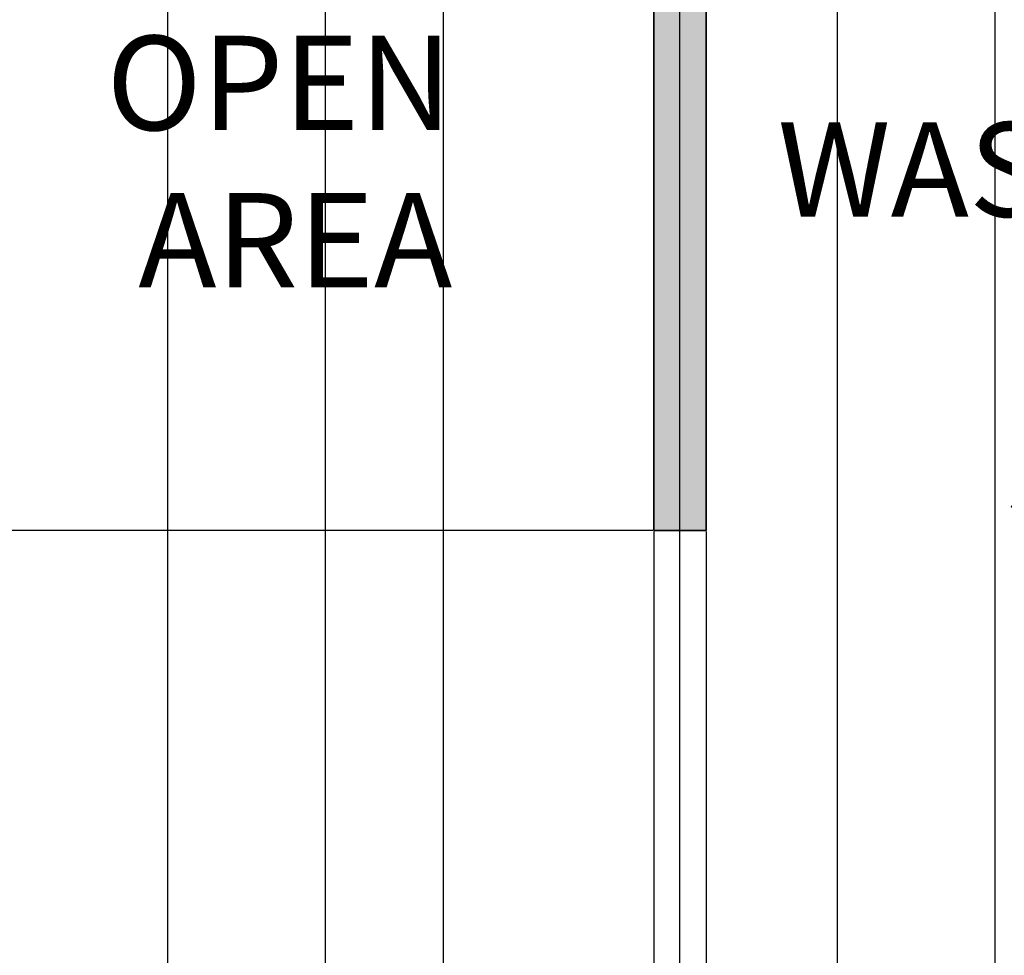
# Model space of a CAD drawing. Units: inches. Extents: x 2103 to 2702, y 2405 to 3142.
# Tile 5 of 7: x 2421 to 2496, y 2968 to 3039. Entities that reach past the tile are written whole.
import ezdxf

# ---------------------------------------------------------------- set-up
doc = ezdxf.new("R2010")
doc.units = ezdxf.units.IN
for name, color, linetype, lineweight in [('A-ANNO-DIMS', 2, 'Continuous', 18), ('A-AREA-IDEN', 7, 'Continuous', 18), ('A-WALL-PATT', 8, 'Continuous', 9), ('WALL', 7, 'Continuous', 35)]:
    doc.layers.add(name, color=color, linetype=linetype, lineweight=lineweight)
doc.styles.get("Standard").update_dxf_attribs({"font": 'arial.ttf'})
doc.dimstyles.get("Standard").update_dxf_attribs({"dimtxt": 9.68, "dimasz": 0.18, "dimexe": 0.18, "dimexo": 0.0625, "dimgap": 0.09, "dimtad": 0, "dimtih": 1, "dimtoh": 1, "dimdec": 1, "dimzin": 0, "dimdsep": 46, "dimlunit": 3, "dimtxsty": 'Standard', "dimcen": 0.09, "dimadec": 0, "dimazin": 0, "dimtfac": 1, "dimtdec": 1, "dimtofl": 0, "dimtmove": 0, "dimatfit": 3, "dimfxl": 1, "dimtolj": 1, "dimtzin": 0, "dimarcsym": 0})

# ---------------------------------------------------------------- blocks, each defined once
blk = doc.blocks.new('*D22')
at = {"layer": 'A-ANNO-DIMS', "color": 0, "lineweight": -2, "transparency": 16777216}
for p, q in [((2342.430135313914, 2939.908174370463), (2342.430135313914, 2945.425674368419)), ((2342.610135313914, 2945.24567436842), (2378.250135313935, 2945.24567436842)), ((2378.430135313934, 2939.90817436637), (2378.430135313934, 2945.425674368419)), ((2378.430135313934, 2945.24567436842), (2378.610135313935, 2945.24567436842))]:
    blk.add_line(p, q, dxfattribs=at)
at = {"layer": 'A-ANNO-DIMS', "color": 0, "transparency": 16777216}
for points in [[(2342.610135313914, 2945.275674368419), (2342.610135313914, 2945.215674368419), (2342.430135313914, 2945.24567436842)], [(2378.250135313935, 2945.275674368419), (2378.250135313935, 2945.215674368419), (2378.430135313934, 2945.24567436842)]]:
    blk.add_solid(points, dxfattribs=at)
at = {"layer": 'Defpoints', "color": 0, "transparency": 16777216}
for p in [(2378.430135313934, 2945.24567436842), (2342.430135313914, 2939.845674370463), (2378.430135313934, 2939.84567436637)]:
    blk.add_point(p, dxfattribs=at)
at = {"layer": 'A-ANNO-DIMS', "color": 0, "transparency": 16777216, "insert": (2453.026820170688, 2945.24567436842), "char_height": 9.68, "attachment_point": 5}
blk.add_mtext('\\A1;ROOM DOOR 3\'-0" TYP.', dxfattribs=at)
blk = doc.blocks.new('*D32')
at = {"layer": 'A-ANNO-DIMS', "color": 0, "lineweight": -2, "transparency": 16777216}
for p, q in [((2523.701954441973, 3069.816092044852), (2527.298623542507, 3072.777740503555)), ((2527.0452500719, 3072.802273835842), (2526.8652500719, 3072.802273835842)), ((2527.15967014106, 3072.663320434396), (2527.0452500719, 3072.802273835842)), ((2546.291633940058, 3049.429184449692), (2527.274090210219, 3072.524367032949)), ((2542.948338310131, 3046.443002658702), (2546.545007410664, 3049.404651117404))]:
    blk.add_line(p, q, dxfattribs=at)
at = {"layer": 'A-ANNO-DIMS', "color": 0, "transparency": 16777216}
for points in [[(2527.297249110461, 3072.543437044476), (2527.250931309978, 3072.505297021422), (2527.15967014106, 3072.663320434396)], [(2546.3147928403, 3049.448254461218), (2546.268475039817, 3049.410114438165), (2546.406054009218, 3049.290231048245)]]:
    blk.add_solid(points, dxfattribs=at)
at = {"layer": 'Defpoints', "color": 0, "transparency": 16777216}
for p in [(2527.15967014106, 3072.663320434396), (2523.653706733137, 3069.776362854172), (2542.900090601295, 3046.403273468022)]:
    blk.add_point(p, dxfattribs=at)
at = {"layer": 'A-ANNO-DIMS', "color": 0, "transparency": 16777216, "insert": (2430.028074082815, 3072.802273835842), "char_height": 9.68, "attachment_point": 5}
blk.add_mtext('\\A1;SINK ENVELOPE 2\'-6 1/2" TYP.', dxfattribs=at)
blk = doc.blocks.new('*D40')
at = {"layer": 'A-ANNO-DIMS', "color": 0, "lineweight": -2, "transparency": 16777216}
for p, q in [((2396.430135, 2906.908174), (2396.430135, 3118.895223)), ((2396.610135, 3118.715223000001), (2407.279400801501, 3118.715223000001)), ((2444.25014, 3118.715223000001), (2433.580874198499, 3118.715223000001)), ((2444.43014, 2842.908175), (2444.43014, 3118.895223))]:
    blk.add_line(p, q, dxfattribs=at)
at = {"layer": 'A-ANNO-DIMS', "color": 0, "transparency": 16777216}
for points in [[(2396.610135, 3118.745223000001), (2396.610135, 3118.685223), (2396.430135, 3118.715223000001)], [(2444.25014, 3118.745223000001), (2444.25014, 3118.685223), (2444.43014, 3118.715223000001)]]:
    blk.add_solid(points, dxfattribs=at)
at = {"layer": 'Defpoints', "color": 0, "transparency": 16777216}
for p in [(2444.43014, 3118.715223000001), (2396.430135, 2906.845674), (2444.43014, 2842.845675)]:
    blk.add_point(p, dxfattribs=at)
at = {"layer": 'A-ANNO-DIMS', "color": 0, "transparency": 16777216, "insert": (2420.4301375, 3118.715223000001), "char_height": 9.68, "attachment_point": 5}
blk.add_mtext('\\A1;4\'-0"', dxfattribs=at)
blk = doc.blocks.new('*D44')
at = {"layer": 'A-ANNO-DIMS', "color": 0, "lineweight": -2, "transparency": 16777216}
for p, q in [((2471.430135, 2560.908174), (2471.430135, 3118.895223)), ((2471.610135, 3118.715223000001), (2483.250135, 3118.715223000001)), ((2483.430135, 2560.908174), (2483.430135, 3118.895223)), ((2483.430135, 3118.715223000001), (2483.610135, 3118.715223000001))]:
    blk.add_line(p, q, dxfattribs=at)
at = {"layer": 'A-ANNO-DIMS', "color": 0, "transparency": 16777216}
for points in [[(2471.610135, 3118.745223000001), (2471.610135, 3118.685223), (2471.430135, 3118.715223000001)], [(2483.250135, 3118.745223000001), (2483.250135, 3118.685223), (2483.430135, 3118.715223000001)]]:
    blk.add_solid(points, dxfattribs=at)
at = {"layer": 'Defpoints', "color": 0, "transparency": 16777216}
for p in [(2483.430135, 3118.715223000001), (2471.430135, 2560.845674), (2483.430135, 2560.845674)]:
    blk.add_point(p, dxfattribs=at)
at = {"layer": 'A-ANNO-DIMS', "color": 0, "transparency": 16777216, "insert": (2496.11047606412, 3118.715223000001), "char_height": 9.68, "attachment_point": 5}
blk.add_mtext('\\A1;1\'-0"', dxfattribs=at)
blk = doc.blocks.new('*D50')
at = {"layer": 'A-ANNO-DIMS', "color": 0, "lineweight": -2, "transparency": 16777216}
for p, q in [((2453.430135, 2569.908174), (2453.430135, 3118.895223)), ((2453.610135, 3118.715223000001), (2461.477488342429, 3118.715223000001)), ((2495.250135, 3118.715223000001), (2487.382781657572, 3118.715223000001)), ((2495.430135, 2569.908174), (2495.430135, 3118.895223))]:
    blk.add_line(p, q, dxfattribs=at)
at = {"layer": 'A-ANNO-DIMS', "color": 0, "transparency": 16777216}
for points in [[(2453.610135, 3118.745223000001), (2453.610135, 3118.685223), (2453.430135, 3118.715223000001)], [(2495.250135, 3118.745223000001), (2495.250135, 3118.685223), (2495.430135, 3118.715223000001)]]:
    blk.add_solid(points, dxfattribs=at)
at = {"layer": 'Defpoints', "color": 0, "transparency": 16777216}
for p in [(2495.430135, 3118.715223000001), (2453.430135, 2569.845674), (2495.430135, 2569.845674)]:
    blk.add_point(p, dxfattribs=at)
at = {"layer": 'A-ANNO-DIMS', "color": 0, "transparency": 16777216, "insert": (2474.430135, 3118.715223000001), "char_height": 9.68, "attachment_point": 5}
blk.add_mtext('\\A1;3\'-6"', dxfattribs=at)
blk = doc.blocks.new('*D66')
at = {"layer": 'A-ANNO-DIMS', "color": 0, "lineweight": -2, "transparency": 16777216}
for p, q in [((2384.430135, 2794.908174), (2384.430135, 3118.895223)), ((2384.610135, 3118.715223000001), (2395.279398301501, 3118.715223000001)), ((2432.250135, 3118.715223000001), (2421.5808716985, 3118.715223000001)), ((2432.430135000001, 2794.908174), (2432.430135000001, 3118.895223))]:
    blk.add_line(p, q, dxfattribs=at)
at = {"layer": 'A-ANNO-DIMS', "color": 0, "transparency": 16777216}
for points in [[(2384.610135, 3118.745223000001), (2384.610135, 3118.685223), (2384.430135, 3118.715223000001)], [(2432.250135, 3118.745223000001), (2432.250135, 3118.685223), (2432.430135000001, 3118.715223000001)]]:
    blk.add_solid(points, dxfattribs=at)
at = {"layer": 'Defpoints', "color": 0, "transparency": 16777216}
for p in [(2384.430135, 3118.715223000001), (2384.430135, 2794.845674), (2432.430135000001, 2794.845674)]:
    blk.add_point(p, dxfattribs=at)
at = {"layer": 'A-ANNO-DIMS', "color": 0, "transparency": 16777216, "insert": (2408.430135, 3118.715223000001), "char_height": 9.68, "attachment_point": 5}
blk.add_mtext('\\A1;4\'-0"', dxfattribs=at)
blk = doc.blocks.new('*D67')
at = {"layer": 'A-ANNO-DIMS', "color": 0, "lineweight": -2, "transparency": 16777216}
for p, q in [((2469.430135, 2999.783174), (2469.430135, 2411.615674)), ((2473.430135, 2999.783174), (2473.430135, 2411.615674)), ((2469.430135, 2411.795674), (2469.250135000001, 2411.795674)), ((2473.250135000001, 2411.795674), (2469.610135, 2411.795674))]:
    blk.add_line(p, q, dxfattribs=at)
at = {"layer": 'A-ANNO-DIMS', "color": 0, "transparency": 16777216}
for points in [[(2469.610135, 2411.825674000001), (2469.610135, 2411.765674), (2469.430135, 2411.795674)], [(2473.250135000001, 2411.825674000001), (2473.250135000001, 2411.765674), (2473.430135, 2411.795674)]]:
    blk.add_solid(points, dxfattribs=at)
at = {"layer": 'Defpoints', "color": 0, "transparency": 16777216}
for p in [(2469.430135, 2999.845674), (2473.430135, 2999.845674), (2469.430135, 2411.795674)]:
    blk.add_point(p, dxfattribs=at)
at = {"layer": 'A-ANNO-DIMS', "color": 0, "transparency": 16777216, "insert": (2456.294186841747, 2411.795674), "char_height": 9.68, "attachment_point": 5}
blk.add_mtext('\\A1;0\'-4"', dxfattribs=at)
blk = doc.blocks.new('*D68')
at = {"layer": 'A-ANNO-DIMS', "color": 0, "lineweight": -2, "transparency": 16777216}
for p, q in [((2469.367635000001, 3059.845674000001), (2211.200134000002, 3059.845674000001)), ((2211.380134000002, 3059.665674000001), (2211.380134000002, 3034.878020521147)), ((2211.380134000002, 3000.025674000001), (2211.380134000002, 3024.813327478856)), ((2469.367635000001, 2999.845674000001), (2211.200134000002, 2999.845674000001))]:
    blk.add_line(p, q, dxfattribs=at)
at = {"layer": 'A-ANNO-DIMS', "color": 0, "transparency": 16777216}
for points in [[(2211.350134000002, 3059.665674000001), (2211.410134000002, 3059.665674000001), (2211.380134000002, 3059.845674000001)], [(2211.350134000002, 3000.025674000001), (2211.410134000002, 3000.025674000001), (2211.380134000002, 2999.845674000001)]]:
    blk.add_solid(points, dxfattribs=at)
at = {"layer": 'Defpoints', "color": 0, "transparency": 16777216}
for p in [(2469.430135000001, 3059.845674000001), (2211.380134000002, 2999.845674000001), (2469.430135000001, 2999.845674000001)]:
    blk.add_point(p, dxfattribs=at)
at = {"layer": 'A-ANNO-DIMS', "color": 0, "transparency": 16777216, "insert": (2211.380134000002, 3029.845674000001), "char_height": 9.68, "attachment_point": 5}
blk.add_mtext('\\A1;5\'-0"', dxfattribs=at)

msp = doc.modelspace()

# ---------------------------------------------------------------- hatches: boundary and pattern name
at = {"layer": 'A-WALL-PATT'}
h = msp.add_hatch(color=256, dxfattribs=at)
h.dxf.hatch_style = 1
h.paths.add_polyline_path([(2255.430135310187, 3059.845674366427), (2289.470134986133, 3059.845674366427), (2289.470134986133, 3068.845673751283), (2289.470134023053, 3068.845673751283), (2246.430135310188, 3068.845674366427), (2246.430135310188, 3024.226823790437), (2255.430135310187, 3024.226823790437)])
h.paths.add_polyline_path([(2408.430135310188, 3068.845674366427), (2337.470134986133, 3068.845674366427), (2337.470134986133, 3059.845674366427), (2387.430135310188, 3059.845674366427), (2387.430135310188, 3035.845674366427), (2387.430135310188, 2915.845674366427), (2378.430135310188, 2915.845674366427), (2378.430135310188, 2906.845674366427), (2396.430135310188, 2906.845674366428), (2396.430135310188, 3059.845674366427), (2408.430135310191, 3059.845674366426), (2408.43013530998, 3063.454696922708)])
h.paths.add_polyline_path([(2482.430134042344, 3068.845674366426), (2456.430135308767, 3068.845674366427), (2456.430135308769, 3059.845674366427), (2469.430135310187, 3059.845674366427), (2469.430135310187, 2999.845674366426), (2473.430135310187, 2999.845674366426), (2473.430135310187, 3003.845674366429), (2473.430135310187, 3059.845674366427), (2482.430134042344, 3059.845674366427)])
h.paths.add_polyline_path([(2606.430135310187, 3068.845674366427), (2506.430135310187, 3068.845674366426), (2506.430135310186, 3059.845674366427), (2533.430135310188, 3059.845674366427), (2533.430135310188, 3045.845674366427), (2533.774306677458, 3045.845674366427, -0.1430353570515649), (2534.312495590746, 3046.002850129938), (2537.430135310188, 3046.002850129938), (2537.430135310188, 3059.845674366427), (2597.430135310188, 3059.845674366427), (2597.430135310187, 3043.845676685565), (2606.430135310187, 3043.845676685565)])

# ---------------------------------------------------------------- linework, layer by layer
at = {"layer": 'WALL'}
for p, q in [((2469.430135310187, 3059.845674366427), (2469.430135310187, 2999.845674366426)), ((2473.430135310187, 3059.845674366427), (2473.430135310187, 3003.845674366429)), ((2473.430135310187, 3003.845674366429), (2473.430135310187, 2999.845674366426)), ((2469.430135310187, 2999.845674366426), (2473.430135310187, 2999.845674366426))]:
    msp.add_line(p, q, dxfattribs=at)

# ---------------------------------------------------------------- texts
at = {"layer": 'A-AREA-IDEN', "char_height": 7.1875, "attachment_point": 3}
for s, insert in [('OPEN AREA{\\H0.83478x; }', (2454.095539138113, 3037.52922569068)), ('WASHING AREA{\\H0.83478x;\\P5\'X9\'4"}', (2523.140832322515, 3030.934615099437))]:
    msp.add_mtext_dynamic_manual_height_columns(s, width=41.38065171367315, gutter_width=12.5, heights=[0], dxfattribs=dict(at, insert=insert))

# ---------------------------------------------------------------- dimensions: what is measured, and where the dimension line sits
at = {"layer": 'A-ANNO-DIMS'}
for base, p1, p2, picture, middle in [((2384.430135, 3118.715223000001), (2432.430135000001, 2794.845674), (2384.430135, 2794.845674), '*D66', (2408.430135, 3118.715223000001)), ((2444.43014, 3118.715223000001), (2396.430135, 2906.845674), (2444.43014, 2842.845675), '*D40', (2420.4301375, 3118.715223000001)), ((2495.430135, 3118.715223000001), (2453.430135, 2569.845674), (2495.430135, 2569.845674), '*D50', (2474.430135, 3118.715223000001)), ((2483.430135, 3118.715223000001), (2471.430135, 2560.845674), (2483.430135, 2560.845674), '*D44', (2496.11047606412, 3118.715223000001)), ((2469.430135, 2411.795674), (2473.430135, 2999.845674), (2469.430135, 2999.845674), '*D67', (2456.294186841747, 2411.795674))]:
    dim = msp.add_linear_dim(base=base, p1=p1, p2=p2, dimstyle='Standard', override={"dimdec": 1, "dimlfac": 1, "dimrnd": 0, "dimzin": 1, "dimdsep": 46, "dimlunit": 4, "dimfrac": 2}, dxfattribs=at)
    dim.commit()
    dim.dimension.update_dxf_attribs({"geometry": picture, "text_midpoint": middle})
for base, p1, p2, angle, text, picture, middle in [((2527.15967014106, 3072.663320434396), (2542.900090601295, 3046.403273468023), (2523.653706733138, 3069.776362854172), 129.4694759592849, 'SINK ENVELOPE <> TYP.', '*D32', (2430.028074082815, 3072.802273835842)), ((2378.430135313934, 2945.24567436842), (2342.430135313914, 2939.845674370463), (2378.430135313934, 2939.84567436637), 359.9999999934862, 'ROOM DOOR <> TYP.', '*D22', (2453.026820170688, 2945.24567436842))]:
    dim = msp.add_linear_dim(base=base, p1=p1, p2=p2, angle=angle, text=text, dimstyle='Standard', override={"dimdec": 1, "dimlfac": 1, "dimrnd": 0, "dimzin": 1, "dimdsep": 46, "dimlunit": 4, "dimfrac": 2}, dxfattribs=at)
    dim.commit()
    dim.dimension.update_dxf_attribs({"geometry": picture, "text_midpoint": middle})
dim = msp.add_linear_dim(base=(2211.380134000002, 2999.845674000001), p1=(2469.430135, 3059.845674), p2=(2469.430135, 2999.845674), angle=90, dimstyle='Standard', override={"dimdec": 1, "dimlfac": 1, "dimrnd": 0, "dimzin": 1, "dimdsep": 46, "dimlunit": 4, "dimfrac": 2}, dxfattribs=at)
dim.commit()
dim.dimension.update_dxf_attribs({"geometry": '*D68', "text_midpoint": (2211.380134000002, 3029.845674000001)})

doc.saveas('drawing.dxf')
